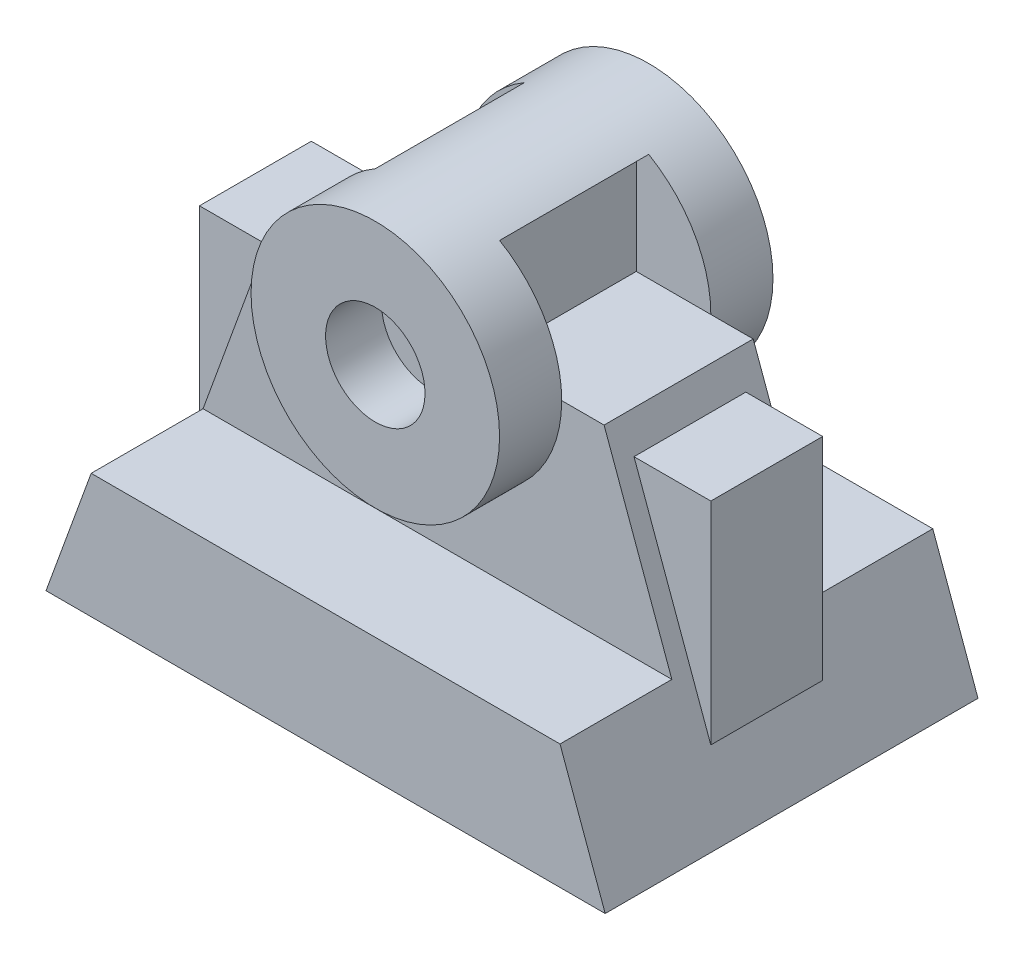
ISO-10303-21;
HEADER;
FILE_DESCRIPTION(('STEP AP214'),'2;1');
FILE_NAME('part.step','',(''),(''),'','','');
FILE_SCHEMA(('AUTOMOTIVE_DESIGN { 1 0 10303 214 1 1 1 1 }'));
ENDSEC;
DATA;
#1=APPLICATION_CONTEXT('core data for automotive mechanical design processes');
#2=APPLICATION_PROTOCOL_DEFINITION('international standard','automotive_design',2000,#1);
#3=PRODUCT_CONTEXT('',#1,'mechanical');
#4=PRODUCT('Part','Part','',(#3));
#5=PRODUCT_RELATED_PRODUCT_CATEGORY('part','',(#4));
#6=PRODUCT_DEFINITION_FORMATION('','',#4);
#7=PRODUCT_DEFINITION_CONTEXT('part definition',#1,'design');
#8=PRODUCT_DEFINITION('design','',#6,#7);
#9=PRODUCT_DEFINITION_SHAPE('','',#8);
#10=(LENGTH_UNIT() NAMED_UNIT(*) SI_UNIT(.MILLI.,.METRE.));
#11=(NAMED_UNIT(*) PLANE_ANGLE_UNIT() SI_UNIT($,.RADIAN.));
#12=(NAMED_UNIT(*) SI_UNIT($,.STERADIAN.) SOLID_ANGLE_UNIT());
#13=UNCERTAINTY_MEASURE_WITH_UNIT(LENGTH_MEASURE(1.E-05),#10,'distance_accuracy_value','');
#14=(GEOMETRIC_REPRESENTATION_CONTEXT(3) GLOBAL_UNCERTAINTY_ASSIGNED_CONTEXT((#13)) GLOBAL_UNIT_ASSIGNED_CONTEXT((#10,
#11,#12)) REPRESENTATION_CONTEXT('',''));
#15=CARTESIAN_POINT('',(0.,0.,0.));
#16=DIRECTION('',(0.,0.,1.));
#17=DIRECTION('',(1.,0.,0.));
#18=AXIS2_PLACEMENT_3D('',#15,#16,#17);
#19=CARTESIAN_POINT('',(45.,50.,7.99999999999999));
#20=DIRECTION('',(0.,0.,1.));
#21=DIRECTION('',(1.,0.,0.));
#22=AXIS2_PLACEMENT_3D('',#19,#20,#21);
#23=CYLINDRICAL_SURFACE('',#22,20.);
#24=CARTESIAN_POINT('',(45.,50.,7.99999999999999));
#25=DIRECTION('',(0.,0.,1.));
#26=DIRECTION('',(1.,0.,0.));
#27=AXIS2_PLACEMENT_3D('',#24,#25,#26);
#28=CIRCLE('',#27,20.);
#29=CARTESIAN_POINT('',(65.,50.,7.99999999999999));
#30=VERTEX_POINT('',#29);
#31=EDGE_CURVE('E315',#30,#30,#28,.T.);
#32=ORIENTED_EDGE('',*,*,#31,.T.);
#33=EDGE_LOOP('',(#32));
#34=FACE_BOUND('',#33,.T.);
#35=CARTESIAN_POINT('',(45.,50.,52.));
#36=DIRECTION('',(0.,0.,1.));
#37=DIRECTION('',(1.,0.,0.));
#38=AXIS2_PLACEMENT_3D('',#35,#36,#37);
#39=CIRCLE('',#38,20.);
#40=CARTESIAN_POINT('',(65.,50.,52.));
#41=VERTEX_POINT('',#40);
#42=EDGE_CURVE('E307',#41,#41,#39,.T.);
#43=ORIENTED_EDGE('',*,*,#42,.F.);
#44=EDGE_LOOP('',(#43));
#45=FACE_BOUND('',#44,.T.);
#46=CARTESIAN_POINT('',(45.,50.,18.));
#47=DIRECTION('',(0.,0.,-1.));
#48=DIRECTION('',(-1.,0.,0.));
#49=AXIS2_PLACEMENT_3D('',#46,#47,#48);
#50=CIRCLE('',#49,20.);
#51=CARTESIAN_POINT('',(65.,50.,18.));
#52=VERTEX_POINT('',#51);
#53=CARTESIAN_POINT('',(25.,50.,18.));
#54=VERTEX_POINT('',#53);
#55=EDGE_CURVE('E320',#52,#54,#50,.T.);
#56=ORIENTED_EDGE('',*,*,#55,.T.);
#57=CARTESIAN_POINT('',(45.,50.,18.));
#58=DIRECTION('',(0.,0.,1.));
#59=DIRECTION('',(1.,0.,0.));
#60=AXIS2_PLACEMENT_3D('',#57,#58,#59);
#61=CIRCLE('',#60,20.);
#62=CARTESIAN_POINT('',(35.,67.3205080756888,18.));
#63=VERTEX_POINT('',#62);
#64=EDGE_CURVE('E11',#54,#63,#61,.F.);
#65=ORIENTED_EDGE('',*,*,#64,.T.);
#66=DIRECTION('',(0.,0.,1.));
#67=VECTOR('',#66,1.);
#68=CARTESIAN_POINT('',(35.,67.3205080756888,7.99999999999999));
#69=LINE('',#68,#67);
#70=CARTESIAN_POINT('',(35.,67.3205080756888,42.));
#71=VERTEX_POINT('',#70);
#72=EDGE_CURVE('E401',#71,#63,#69,.F.);
#73=ORIENTED_EDGE('',*,*,#72,.F.);
#74=CARTESIAN_POINT('',(45.,50.,42.));
#75=DIRECTION('',(0.,0.,-1.));
#76=DIRECTION('',(-1.,0.,0.));
#77=AXIS2_PLACEMENT_3D('',#74,#75,#76);
#78=CIRCLE('',#77,20.);
#79=CARTESIAN_POINT('',(25.,50.,42.));
#80=VERTEX_POINT('',#79);
#81=EDGE_CURVE('E52',#71,#80,#78,.F.);
#82=ORIENTED_EDGE('',*,*,#81,.T.);
#83=CARTESIAN_POINT('',(45.,50.,42.));
#84=DIRECTION('',(0.,0.,1.));
#85=DIRECTION('',(1.,0.,0.));
#86=AXIS2_PLACEMENT_3D('',#83,#84,#85);
#87=CIRCLE('',#86,20.);
#88=CARTESIAN_POINT('',(65.,50.,42.));
#89=VERTEX_POINT('',#88);
#90=EDGE_CURVE('E308',#80,#89,#87,.T.);
#91=ORIENTED_EDGE('',*,*,#90,.T.);
#92=CARTESIAN_POINT('',(45.,50.,42.));
#93=DIRECTION('',(0.,0.,1.));
#94=DIRECTION('',(1.,0.,0.));
#95=AXIS2_PLACEMENT_3D('',#92,#93,#94);
#96=CIRCLE('',#95,20.);
#97=CARTESIAN_POINT('',(55.,67.3205080756888,42.));
#98=VERTEX_POINT('',#97);
#99=EDGE_CURVE('E217',#98,#89,#96,.F.);
#100=ORIENTED_EDGE('',*,*,#99,.F.);
#101=DIRECTION('',(0.,0.,1.));
#102=VECTOR('',#101,1.);
#103=CARTESIAN_POINT('',(55.,67.3205080756888,7.99999999999999));
#104=LINE('',#103,#102);
#105=CARTESIAN_POINT('',(55.,67.3205080756888,18.));
#106=VERTEX_POINT('',#105);
#107=EDGE_CURVE('E396',#106,#98,#104,.T.);
#108=ORIENTED_EDGE('',*,*,#107,.F.);
#109=CARTESIAN_POINT('',(45.,50.,18.));
#110=DIRECTION('',(0.,0.,-1.));
#111=DIRECTION('',(0.,1.,0.));
#112=AXIS2_PLACEMENT_3D('',#109,#110,#111);
#113=CIRCLE('',#112,20.);
#114=EDGE_CURVE('E397',#52,#106,#113,.F.);
#115=ORIENTED_EDGE('',*,*,#114,.F.);
#116=EDGE_LOOP('',(#56,#65,#73,#82,#91,#100,#108,#115));
#117=FACE_BOUND('',#116,.T.);
#118=ADVANCED_FACE('F44',(#34,#45,#117),#23,.T.);
#119=CARTESIAN_POINT('',(20.,55.,18.));
#120=DIRECTION('',(-0.939793423488437,0.341743063086705,0.));
#121=DIRECTION('',(-0.341743063086705,-0.939793423488437,0.));
#122=AXIS2_PLACEMENT_3D('',#119,#120,#121);
#123=PLANE('',#122);
#124=DIRECTION('',(0.,0.,1.));
#125=VECTOR('',#124,1.);
#126=CARTESIAN_POINT('',(18.1818181818182,50.,18.));
#127=LINE('',#126,#125);
#128=CARTESIAN_POINT('',(18.1818181818182,50.,18.));
#129=VERTEX_POINT('',#128);
#130=CARTESIAN_POINT('',(18.1818181818182,50.,42.));
#131=VERTEX_POINT('',#130);
#132=EDGE_CURVE('E342',#129,#131,#127,.T.);
#133=ORIENTED_EDGE('',*,*,#132,.F.);
#134=DIRECTION('',(-0.341743063086705,-0.939793423488437,0.));
#135=VECTOR('',#134,1.);
#136=CARTESIAN_POINT('',(20.,55.,18.));
#137=LINE('',#136,#135);
#138=CARTESIAN_POINT('',(7.27272727272728,20.,18.));
#139=VERTEX_POINT('',#138);
#140=EDGE_CURVE('E364',#129,#139,#137,.T.);
#141=ORIENTED_EDGE('',*,*,#140,.T.);
#142=DIRECTION('',(0.,0.,1.));
#143=VECTOR('',#142,1.);
#144=CARTESIAN_POINT('',(7.27272727272728,20.,0.));
#145=LINE('',#144,#143);
#146=CARTESIAN_POINT('',(7.27272727272728,20.,0.));
#147=VERTEX_POINT('',#146);
#148=EDGE_CURVE('E328',#147,#139,#145,.T.);
#149=ORIENTED_EDGE('',*,*,#148,.F.);
#150=DIRECTION('',(-0.341743063086704,-0.939793423488437,0.));
#151=VECTOR('',#150,1.);
#152=CARTESIAN_POINT('',(0.,0.,0.));
#153=LINE('',#152,#151);
#154=CARTESIAN_POINT('',(0.,0.,0.));
#155=VERTEX_POINT('',#154);
#156=EDGE_CURVE('E323',#147,#155,#153,.T.);
#157=ORIENTED_EDGE('',*,*,#156,.T.);
#158=DIRECTION('',(0.,0.,-1.));
#159=VECTOR('',#158,1.);
#160=CARTESIAN_POINT('',(0.,0.,60.));
#161=LINE('',#160,#159);
#162=CARTESIAN_POINT('',(0.,0.,60.));
#163=VERTEX_POINT('',#162);
#164=EDGE_CURVE('E382',#163,#155,#161,.T.);
#165=ORIENTED_EDGE('',*,*,#164,.F.);
#166=DIRECTION('',(-0.341743063086704,-0.939793423488437,0.));
#167=VECTOR('',#166,1.);
#168=CARTESIAN_POINT('',(0.,0.,60.));
#169=LINE('',#168,#167);
#170=CARTESIAN_POINT('',(7.27272727272728,20.,60.));
#171=VERTEX_POINT('',#170);
#172=EDGE_CURVE('E324',#171,#163,#169,.T.);
#173=ORIENTED_EDGE('',*,*,#172,.F.);
#174=CARTESIAN_POINT('',(7.27272727272728,20.,42.));
#175=VERTEX_POINT('',#174);
#176=EDGE_CURVE('E321',#175,#171,#145,.T.);
#177=ORIENTED_EDGE('',*,*,#176,.F.);
#178=DIRECTION('',(-0.341743063086705,-0.939793423488437,0.));
#179=VECTOR('',#178,1.);
#180=CARTESIAN_POINT('',(7.27272727272728,20.,42.));
#181=LINE('',#180,#179);
#182=EDGE_CURVE('E354',#131,#175,#181,.T.);
#183=ORIENTED_EDGE('',*,*,#182,.F.);
#184=EDGE_LOOP('',(#133,#141,#149,#157,#165,#173,#177,#183));
#185=FACE_BOUND('',#184,.T.);
#186=DIRECTION('',(0.341743063086705,0.939793423488437,0.));
#187=VECTOR('',#186,1.);
#188=CARTESIAN_POINT('',(20.,55.,21.));
#189=LINE('',#188,#187);
#190=CARTESIAN_POINT('',(3.63636363636363,9.99999999999999,21.));
#191=VERTEX_POINT('',#190);
#192=CARTESIAN_POINT('',(3.7,10.175,21.));
#193=VERTEX_POINT('',#192);
#194=EDGE_CURVE('E301',#191,#193,#189,.T.);
#195=ORIENTED_EDGE('',*,*,#194,.T.);
#196=CARTESIAN_POINT('',(16.3636363636364,45.,21.));
#197=VERTEX_POINT('',#196);
#198=EDGE_CURVE('E68',#193,#197,#189,.T.);
#199=ORIENTED_EDGE('',*,*,#198,.T.);
#200=DIRECTION('',(0.,0.,1.));
#201=VECTOR('',#200,1.);
#202=CARTESIAN_POINT('',(16.3636363636364,45.,18.));
#203=LINE('',#202,#201);
#204=CARTESIAN_POINT('',(16.3636363636364,45.,39.));
#205=VERTEX_POINT('',#204);
#206=EDGE_CURVE('E306',#197,#205,#203,.T.);
#207=ORIENTED_EDGE('',*,*,#206,.T.);
#208=DIRECTION('',(-0.341743063086705,-0.939793423488437,0.));
#209=VECTOR('',#208,1.);
#210=CARTESIAN_POINT('',(20.,55.,39.));
#211=LINE('',#210,#209);
#212=CARTESIAN_POINT('',(3.7,10.175,39.));
#213=VERTEX_POINT('',#212);
#214=EDGE_CURVE('E303',#205,#213,#211,.T.);
#215=ORIENTED_EDGE('',*,*,#214,.T.);
#216=DIRECTION('',(0.341743063086705,0.939793423488437,0.));
#217=VECTOR('',#216,1.);
#218=CARTESIAN_POINT('',(20.,55.,39.));
#219=LINE('',#218,#217);
#220=CARTESIAN_POINT('',(3.63636363636363,9.99999999999999,39.));
#221=VERTEX_POINT('',#220);
#222=EDGE_CURVE('E285',#221,#213,#219,.T.);
#223=ORIENTED_EDGE('',*,*,#222,.F.);
#224=DIRECTION('',(0.,0.,-1.));
#225=VECTOR('',#224,1.);
#226=CARTESIAN_POINT('',(3.63636363636363,9.99999999999999,18.));
#227=LINE('',#226,#225);
#228=EDGE_CURVE('E393',#221,#191,#227,.T.);
#229=ORIENTED_EDGE('',*,*,#228,.T.);
#230=EDGE_LOOP('',(#195,#199,#207,#215,#223,#229));
#231=FACE_BOUND('',#230,.T.);
#232=ADVANCED_FACE('F440',(#185,#231),#123,.T.);
#233=CARTESIAN_POINT('',(70.,55.,18.));
#234=DIRECTION('',(0.939793423488437,0.341743063086704,0.));
#235=DIRECTION('',(-0.341743063086704,0.939793423488437,0.));
#236=AXIS2_PLACEMENT_3D('',#233,#234,#235);
#237=PLANE('',#236);
#238=DIRECTION('',(0.,0.,1.));
#239=VECTOR('',#238,1.);
#240=CARTESIAN_POINT('',(71.8181818181818,50.,18.));
#241=LINE('',#240,#239);
#242=CARTESIAN_POINT('',(71.8181818181818,50.,18.));
#243=VERTEX_POINT('',#242);
#244=CARTESIAN_POINT('',(71.8181818181818,50.,42.));
#245=VERTEX_POINT('',#244);
#246=EDGE_CURVE('E338',#243,#245,#241,.T.);
#247=ORIENTED_EDGE('',*,*,#246,.T.);
#248=DIRECTION('',(-0.341743063086704,0.939793423488437,0.));
#249=VECTOR('',#248,1.);
#250=CARTESIAN_POINT('',(70.,55.,42.));
#251=LINE('',#250,#249);
#252=CARTESIAN_POINT('',(82.7272727272727,20.,42.));
#253=VERTEX_POINT('',#252);
#254=EDGE_CURVE('E355',#253,#245,#251,.T.);
#255=ORIENTED_EDGE('',*,*,#254,.F.);
#256=DIRECTION('',(0.,0.,1.));
#257=VECTOR('',#256,1.);
#258=CARTESIAN_POINT('',(82.7272727272727,20.,0.));
#259=LINE('',#258,#257);
#260=CARTESIAN_POINT('',(82.7272727272727,20.,60.));
#261=VERTEX_POINT('',#260);
#262=EDGE_CURVE('E332',#253,#261,#259,.T.);
#263=ORIENTED_EDGE('',*,*,#262,.T.);
#264=DIRECTION('',(0.341743063086704,-0.939793423488437,0.));
#265=VECTOR('',#264,1.);
#266=CARTESIAN_POINT('',(79.4890510948905,28.9051094890511,60.));
#267=LINE('',#266,#265);
#268=CARTESIAN_POINT('',(90.,0.,60.));
#269=VERTEX_POINT('',#268);
#270=EDGE_CURVE('E318',#261,#269,#267,.T.);
#271=ORIENTED_EDGE('',*,*,#270,.T.);
#272=DIRECTION('',(0.,0.,-1.));
#273=VECTOR('',#272,1.);
#274=CARTESIAN_POINT('',(90.,0.,60.));
#275=LINE('',#274,#273);
#276=CARTESIAN_POINT('',(90.,0.,0.));
#277=VERTEX_POINT('',#276);
#278=EDGE_CURVE('E374',#269,#277,#275,.T.);
#279=ORIENTED_EDGE('',*,*,#278,.T.);
#280=DIRECTION('',(0.341743063086704,-0.939793423488437,0.));
#281=VECTOR('',#280,1.);
#282=CARTESIAN_POINT('',(79.4890510948905,28.9051094890511,0.));
#283=LINE('',#282,#281);
#284=CARTESIAN_POINT('',(82.7272727272727,20.,0.));
#285=VERTEX_POINT('',#284);
#286=EDGE_CURVE('E331',#285,#277,#283,.T.);
#287=ORIENTED_EDGE('',*,*,#286,.F.);
#288=CARTESIAN_POINT('',(82.7272727272727,20.,18.));
#289=VERTEX_POINT('',#288);
#290=EDGE_CURVE('E330',#285,#289,#259,.T.);
#291=ORIENTED_EDGE('',*,*,#290,.T.);
#292=DIRECTION('',(-0.341743063086704,0.939793423488437,0.));
#293=VECTOR('',#292,1.);
#294=CARTESIAN_POINT('',(70.,55.,18.));
#295=LINE('',#294,#293);
#296=EDGE_CURVE('E363',#289,#243,#295,.T.);
#297=ORIENTED_EDGE('',*,*,#296,.T.);
#298=EDGE_LOOP('',(#247,#255,#263,#271,#279,#287,#291,#297));
#299=FACE_BOUND('',#298,.T.);
#300=DIRECTION('',(-0.341743063086704,0.939793423488437,0.));
#301=VECTOR('',#300,1.);
#302=CARTESIAN_POINT('',(70.,55.,39.));
#303=LINE('',#302,#301);
#304=CARTESIAN_POINT('',(86.,11.,39.));
#305=VERTEX_POINT('',#304);
#306=CARTESIAN_POINT('',(73.6363636363637,45.,39.));
#307=VERTEX_POINT('',#306);
#308=EDGE_CURVE('E389',#305,#307,#303,.T.);
#309=ORIENTED_EDGE('',*,*,#308,.T.);
#310=DIRECTION('',(0.,0.,-1.));
#311=VECTOR('',#310,1.);
#312=CARTESIAN_POINT('',(73.6363636363637,45.,18.));
#313=LINE('',#312,#311);
#314=CARTESIAN_POINT('',(73.6363636363637,45.,21.));
#315=VERTEX_POINT('',#314);
#316=EDGE_CURVE('E392',#307,#315,#313,.T.);
#317=ORIENTED_EDGE('',*,*,#316,.T.);
#318=DIRECTION('',(0.341743063086704,-0.939793423488437,0.));
#319=VECTOR('',#318,1.);
#320=CARTESIAN_POINT('',(70.,55.,21.));
#321=LINE('',#320,#319);
#322=CARTESIAN_POINT('',(86.,11.,21.));
#323=VERTEX_POINT('',#322);
#324=EDGE_CURVE('E390',#315,#323,#321,.T.);
#325=ORIENTED_EDGE('',*,*,#324,.T.);
#326=DIRECTION('',(0.,0.,-1.));
#327=VECTOR('',#326,1.);
#328=CARTESIAN_POINT('',(86.,11.,18.));
#329=LINE('',#328,#327);
#330=EDGE_CURVE('E381',#305,#323,#329,.T.);
#331=ORIENTED_EDGE('',*,*,#330,.F.);
#332=EDGE_LOOP('',(#309,#317,#325,#331));
#333=FACE_BOUND('',#332,.T.);
#334=ADVANCED_FACE('F421',(#299,#333),#237,.T.);
#335=CARTESIAN_POINT('',(0.,0.,42.));
#336=DIRECTION('',(0.,0.,-1.));
#337=DIRECTION('',(-1.,0.,0.));
#338=AXIS2_PLACEMENT_3D('',#335,#336,#337);
#339=PLANE('',#338);
#340=ORIENTED_EDGE('',*,*,#90,.F.);
#341=DIRECTION('',(1.,0.,0.));
#342=VECTOR('',#341,1.);
#343=CARTESIAN_POINT('',(45.,50.,42.));
#344=LINE('',#343,#342);
#345=EDGE_CURVE('E345',#131,#80,#344,.T.);
#346=ORIENTED_EDGE('',*,*,#345,.F.);
#347=ORIENTED_EDGE('',*,*,#182,.T.);
#348=DIRECTION('',(1.,0.,0.));
#349=VECTOR('',#348,1.);
#350=CARTESIAN_POINT('',(82.7272727272727,20.,42.));
#351=LINE('',#350,#349);
#352=EDGE_CURVE('E350',#175,#253,#351,.T.);
#353=ORIENTED_EDGE('',*,*,#352,.T.);
#354=ORIENTED_EDGE('',*,*,#254,.T.);
#355=EDGE_CURVE('E326',#89,#245,#344,.T.);
#356=ORIENTED_EDGE('',*,*,#355,.F.);
#357=EDGE_LOOP('',(#340,#346,#347,#353,#354,#356));
#358=FACE_BOUND('',#357,.T.);
#359=ADVANCED_FACE('F417',(#358),#339,.F.);
#360=CARTESIAN_POINT('',(45.,50.,18.));
#361=DIRECTION('',(0.,-1.,0.));
#362=DIRECTION('',(0.,0.,-1.));
#363=AXIS2_PLACEMENT_3D('',#360,#361,#362);
#364=PLANE('',#363);
#365=DIRECTION('',(1.,0.,0.));
#366=VECTOR('',#365,1.);
#367=CARTESIAN_POINT('',(45.,50.,18.));
#368=LINE('',#367,#366);
#369=EDGE_CURVE('E343',#52,#243,#368,.T.);
#370=ORIENTED_EDGE('',*,*,#369,.F.);
#371=DIRECTION('',(1.,0.,0.));
#372=VECTOR('',#371,1.);
#373=CARTESIAN_POINT('',(55.,50.,18.));
#374=LINE('',#373,#372);
#375=CARTESIAN_POINT('',(53.,50.,18.));
#376=VERTEX_POINT('',#375);
#377=EDGE_CURVE('E219',#376,#52,#374,.T.);
#378=ORIENTED_EDGE('',*,*,#377,.F.);
#379=DIRECTION('',(0.,0.,-1.));
#380=VECTOR('',#379,1.);
#381=CARTESIAN_POINT('',(53.,50.,18.));
#382=LINE('',#381,#380);
#383=CARTESIAN_POINT('',(53.,50.,42.));
#384=VERTEX_POINT('',#383);
#385=EDGE_CURVE('E223',#384,#376,#382,.T.);
#386=ORIENTED_EDGE('',*,*,#385,.F.);
#387=DIRECTION('',(1.,0.,0.));
#388=VECTOR('',#387,1.);
#389=CARTESIAN_POINT('',(55.,50.,42.));
#390=LINE('',#389,#388);
#391=EDGE_CURVE('E209',#384,#89,#390,.T.);
#392=ORIENTED_EDGE('',*,*,#391,.T.);
#393=ORIENTED_EDGE('',*,*,#355,.T.);
#394=ORIENTED_EDGE('',*,*,#246,.F.);
#395=EDGE_LOOP('',(#370,#378,#386,#392,#393,#394));
#396=FACE_BOUND('',#395,.T.);
#397=ADVANCED_FACE('F224',(#396),#364,.F.);
#398=CARTESIAN_POINT('',(90.,20.,60.));
#399=DIRECTION('',(0.,-1.,0.));
#400=DIRECTION('',(0.,0.,-1.));
#401=AXIS2_PLACEMENT_3D('',#398,#399,#400);
#402=PLANE('',#401);
#403=ORIENTED_EDGE('',*,*,#176,.T.);
#404=DIRECTION('',(-1.,0.,0.));
#405=VECTOR('',#404,1.);
#406=CARTESIAN_POINT('',(90.,20.,60.));
#407=LINE('',#406,#405);
#408=EDGE_CURVE('E371',#261,#171,#407,.T.);
#409=ORIENTED_EDGE('',*,*,#408,.F.);
#410=ORIENTED_EDGE('',*,*,#262,.F.);
#411=ORIENTED_EDGE('',*,*,#352,.F.);
#412=EDGE_LOOP('',(#403,#409,#410,#411));
#413=FACE_BOUND('',#412,.T.);
#414=ADVANCED_FACE('F484',(#413),#402,.F.);
#415=ORIENTED_EDGE('',*,*,#148,.T.);
#416=DIRECTION('',(1.,0.,0.));
#417=VECTOR('',#416,1.);
#418=CARTESIAN_POINT('',(45.,20.,18.));
#419=LINE('',#418,#417);
#420=EDGE_CURVE('E356',#139,#289,#419,.T.);
#421=ORIENTED_EDGE('',*,*,#420,.T.);
#422=ORIENTED_EDGE('',*,*,#290,.F.);
#423=DIRECTION('',(-1.,0.,0.));
#424=VECTOR('',#423,1.);
#425=CARTESIAN_POINT('',(90.,20.,0.));
#426=LINE('',#425,#424);
#427=EDGE_CURVE('E375',#285,#147,#426,.T.);
#428=ORIENTED_EDGE('',*,*,#427,.T.);
#429=EDGE_LOOP('',(#415,#421,#422,#428));
#430=FACE_BOUND('',#429,.T.);
#431=ADVANCED_FACE('F433',(#430),#402,.F.);
#432=CARTESIAN_POINT('',(0.,0.,60.));
#433=DIRECTION('',(0.,0.,1.));
#434=DIRECTION('',(1.,0.,0.));
#435=AXIS2_PLACEMENT_3D('',#432,#433,#434);
#436=PLANE('',#435);
#437=ORIENTED_EDGE('',*,*,#408,.T.);
#438=ORIENTED_EDGE('',*,*,#172,.T.);
#439=DIRECTION('',(1.,0.,0.));
#440=VECTOR('',#439,1.);
#441=CARTESIAN_POINT('',(0.,0.,60.));
#442=LINE('',#441,#440);
#443=EDGE_CURVE('E368',#163,#269,#442,.T.);
#444=ORIENTED_EDGE('',*,*,#443,.T.);
#445=ORIENTED_EDGE('',*,*,#270,.F.);
#446=EDGE_LOOP('',(#437,#438,#444,#445));
#447=FACE_BOUND('',#446,.T.);
#448=ADVANCED_FACE('F478',(#447),#436,.T.);
#449=CARTESIAN_POINT('',(0.,0.,0.));
#450=DIRECTION('',(0.,0.,1.));
#451=DIRECTION('',(1.,0.,0.));
#452=AXIS2_PLACEMENT_3D('',#449,#450,#451);
#453=PLANE('',#452);
#454=ORIENTED_EDGE('',*,*,#156,.F.);
#455=ORIENTED_EDGE('',*,*,#427,.F.);
#456=ORIENTED_EDGE('',*,*,#286,.T.);
#457=DIRECTION('',(1.,0.,0.));
#458=VECTOR('',#457,1.);
#459=CARTESIAN_POINT('',(0.,0.,0.));
#460=LINE('',#459,#458);
#461=EDGE_CURVE('E370',#155,#277,#460,.T.);
#462=ORIENTED_EDGE('',*,*,#461,.F.);
#463=EDGE_LOOP('',(#454,#455,#456,#462));
#464=FACE_BOUND('',#463,.T.);
#465=ADVANCED_FACE('F481',(#464),#453,.F.);
#466=CARTESIAN_POINT('',(0.,0.,60.));
#467=DIRECTION('',(0.,1.,0.));
#468=DIRECTION('',(0.,0.,1.));
#469=AXIS2_PLACEMENT_3D('',#466,#467,#468);
#470=PLANE('',#469);
#471=ORIENTED_EDGE('',*,*,#461,.T.);
#472=ORIENTED_EDGE('',*,*,#278,.F.);
#473=ORIENTED_EDGE('',*,*,#443,.F.);
#474=ORIENTED_EDGE('',*,*,#164,.T.);
#475=EDGE_LOOP('',(#471,#472,#473,#474));
#476=FACE_BOUND('',#475,.T.);
#477=ADVANCED_FACE('F50',(#476),#470,.F.);
#478=CARTESIAN_POINT('',(0.,0.,18.));
#479=DIRECTION('',(0.,0.,-1.));
#480=DIRECTION('',(-1.,0.,0.));
#481=AXIS2_PLACEMENT_3D('',#478,#479,#480);
#482=PLANE('',#481);
#483=ORIENTED_EDGE('',*,*,#55,.F.);
#484=ORIENTED_EDGE('',*,*,#369,.T.);
#485=ORIENTED_EDGE('',*,*,#296,.F.);
#486=ORIENTED_EDGE('',*,*,#420,.F.);
#487=ORIENTED_EDGE('',*,*,#140,.F.);
#488=EDGE_CURVE('E340',#129,#54,#368,.T.);
#489=ORIENTED_EDGE('',*,*,#488,.T.);
#490=EDGE_LOOP('',(#483,#484,#485,#486,#487,#489));
#491=FACE_BOUND('',#490,.T.);
#492=ADVANCED_FACE('F427',(#491),#482,.T.);
#493=ORIENTED_EDGE('',*,*,#345,.T.);
#494=DIRECTION('',(-1.,0.,0.));
#495=VECTOR('',#494,1.);
#496=CARTESIAN_POINT('',(35.,50.,42.));
#497=LINE('',#496,#495);
#498=CARTESIAN_POINT('',(37.,50.,42.));
#499=VERTEX_POINT('',#498);
#500=EDGE_CURVE('E265',#499,#80,#497,.T.);
#501=ORIENTED_EDGE('',*,*,#500,.F.);
#502=DIRECTION('',(0.,0.,1.));
#503=VECTOR('',#502,1.);
#504=CARTESIAN_POINT('',(37.,50.,42.));
#505=LINE('',#504,#503);
#506=CARTESIAN_POINT('',(37.,50.,18.));
#507=VERTEX_POINT('',#506);
#508=EDGE_CURVE('E249',#507,#499,#505,.T.);
#509=ORIENTED_EDGE('',*,*,#508,.F.);
#510=DIRECTION('',(-1.,0.,0.));
#511=VECTOR('',#510,1.);
#512=CARTESIAN_POINT('',(35.,50.,18.));
#513=LINE('',#512,#511);
#514=EDGE_CURVE('E216',#507,#54,#513,.T.);
#515=ORIENTED_EDGE('',*,*,#514,.T.);
#516=ORIENTED_EDGE('',*,*,#488,.F.);
#517=ORIENTED_EDGE('',*,*,#132,.T.);
#518=EDGE_LOOP('',(#493,#501,#509,#515,#516,#517));
#519=FACE_BOUND('',#518,.T.);
#520=ADVANCED_FACE('F413',(#519),#364,.F.);
#521=CARTESIAN_POINT('',(45.,50.,7.99999999999999));
#522=DIRECTION('',(0.,0.,1.));
#523=DIRECTION('',(1.,0.,0.));
#524=AXIS2_PLACEMENT_3D('',#521,#522,#523);
#525=PLANE('',#524);
#526=CARTESIAN_POINT('',(45.,50.,7.99999999999999));
#527=DIRECTION('',(0.,0.,-1.));
#528=DIRECTION('',(-1.,0.,0.));
#529=AXIS2_PLACEMENT_3D('',#526,#527,#528);
#530=CIRCLE('',#529,8.00000000000001);
#531=CARTESIAN_POINT('',(37.,50.,7.99999999999999));
#532=VERTEX_POINT('',#531);
#533=EDGE_CURVE('E908',#532,#532,#530,.T.);
#534=ORIENTED_EDGE('',*,*,#533,.F.);
#535=EDGE_LOOP('',(#534));
#536=FACE_BOUND('',#535,.T.);
#537=ORIENTED_EDGE('',*,*,#31,.F.);
#538=EDGE_LOOP('',(#537));
#539=FACE_BOUND('',#538,.T.);
#540=ADVANCED_FACE('F466',(#536,#539),#525,.F.);
#541=CARTESIAN_POINT('',(45.,50.,52.));
#542=DIRECTION('',(0.,0.,1.));
#543=DIRECTION('',(1.,0.,0.));
#544=AXIS2_PLACEMENT_3D('',#541,#542,#543);
#545=PLANE('',#544);
#546=CARTESIAN_POINT('',(45.,50.,52.));
#547=DIRECTION('',(0.,0.,1.));
#548=DIRECTION('',(1.,0.,0.));
#549=AXIS2_PLACEMENT_3D('',#546,#547,#548);
#550=CIRCLE('',#549,8.);
#551=CARTESIAN_POINT('',(53.,50.,52.));
#552=VERTEX_POINT('',#551);
#553=EDGE_CURVE('E240',#552,#552,#550,.T.);
#554=ORIENTED_EDGE('',*,*,#553,.F.);
#555=EDGE_LOOP('',(#554));
#556=FACE_BOUND('',#555,.T.);
#557=ORIENTED_EDGE('',*,*,#42,.T.);
#558=EDGE_LOOP('',(#557));
#559=FACE_BOUND('',#558,.T.);
#560=ADVANCED_FACE('F523',(#556,#559),#545,.T.);
#561=CARTESIAN_POINT('',(86.,0.,0.));
#562=DIRECTION('',(1.,0.,0.));
#563=DIRECTION('',(0.,0.,-1.));
#564=AXIS2_PLACEMENT_3D('',#561,#562,#563);
#565=PLANE('',#564);
#566=DIRECTION('',(0.,-1.,0.));
#567=VECTOR('',#566,1.);
#568=CARTESIAN_POINT('',(86.,45.,39.));
#569=LINE('',#568,#567);
#570=CARTESIAN_POINT('',(86.,45.,39.));
#571=VERTEX_POINT('',#570);
#572=EDGE_CURVE('E288',#571,#305,#569,.T.);
#573=ORIENTED_EDGE('',*,*,#572,.T.);
#574=ORIENTED_EDGE('',*,*,#330,.T.);
#575=DIRECTION('',(0.,1.,0.));
#576=VECTOR('',#575,1.);
#577=CARTESIAN_POINT('',(86.,9.99999999999999,21.));
#578=LINE('',#577,#576);
#579=CARTESIAN_POINT('',(86.,45.,21.));
#580=VERTEX_POINT('',#579);
#581=EDGE_CURVE('E293',#323,#580,#578,.T.);
#582=ORIENTED_EDGE('',*,*,#581,.T.);
#583=DIRECTION('',(0.,0.,1.));
#584=VECTOR('',#583,1.);
#585=CARTESIAN_POINT('',(86.,45.,21.));
#586=LINE('',#585,#584);
#587=EDGE_CURVE('E286',#580,#571,#586,.T.);
#588=ORIENTED_EDGE('',*,*,#587,.T.);
#589=EDGE_LOOP('',(#573,#574,#582,#588));
#590=FACE_BOUND('',#589,.T.);
#591=ADVANCED_FACE('F518',(#590),#565,.T.);
#592=CARTESIAN_POINT('',(86.,9.99999999999999,21.));
#593=DIRECTION('',(0.,0.,1.));
#594=DIRECTION('',(1.,0.,0.));
#595=AXIS2_PLACEMENT_3D('',#592,#593,#594);
#596=PLANE('',#595);
#597=ORIENTED_EDGE('',*,*,#324,.F.);
#598=DIRECTION('',(-1.,0.,0.));
#599=VECTOR('',#598,1.);
#600=CARTESIAN_POINT('',(86.,45.,21.));
#601=LINE('',#600,#599);
#602=EDGE_CURVE('E295',#580,#315,#601,.T.);
#603=ORIENTED_EDGE('',*,*,#602,.F.);
#604=ORIENTED_EDGE('',*,*,#581,.F.);
#605=EDGE_LOOP('',(#597,#603,#604));
#606=FACE_BOUND('',#605,.T.);
#607=ADVANCED_FACE('F525',(#606),#596,.F.);
#608=CARTESIAN_POINT('',(86.,45.,39.));
#609=DIRECTION('',(0.,0.,-1.));
#610=DIRECTION('',(-1.,0.,0.));
#611=AXIS2_PLACEMENT_3D('',#608,#609,#610);
#612=PLANE('',#611);
#613=ORIENTED_EDGE('',*,*,#308,.F.);
#614=ORIENTED_EDGE('',*,*,#572,.F.);
#615=DIRECTION('',(-1.,0.,0.));
#616=VECTOR('',#615,1.);
#617=CARTESIAN_POINT('',(86.,45.,39.));
#618=LINE('',#617,#616);
#619=EDGE_CURVE('E296',#571,#307,#618,.T.);
#620=ORIENTED_EDGE('',*,*,#619,.T.);
#621=EDGE_LOOP('',(#613,#614,#620));
#622=FACE_BOUND('',#621,.T.);
#623=ADVANCED_FACE('F540',(#622),#612,.F.);
#624=CARTESIAN_POINT('',(86.,45.,30.));
#625=DIRECTION('',(0.,-1.,0.));
#626=DIRECTION('',(0.,0.,-1.));
#627=AXIS2_PLACEMENT_3D('',#624,#625,#626);
#628=PLANE('',#627);
#629=ORIENTED_EDGE('',*,*,#316,.F.);
#630=ORIENTED_EDGE('',*,*,#619,.F.);
#631=ORIENTED_EDGE('',*,*,#587,.F.);
#632=ORIENTED_EDGE('',*,*,#602,.T.);
#633=EDGE_LOOP('',(#629,#630,#631,#632));
#634=FACE_BOUND('',#633,.T.);
#635=ADVANCED_FACE('F549',(#634),#628,.F.);
#636=CARTESIAN_POINT('',(3.69999999999999,45.,21.));
#637=VERTEX_POINT('',#636);
#638=EDGE_CURVE('E291',#197,#637,#601,.T.);
#639=ORIENTED_EDGE('',*,*,#638,.T.);
#640=DIRECTION('',(0.,0.,-1.));
#641=VECTOR('',#640,1.);
#642=CARTESIAN_POINT('',(3.7,45.,21.));
#643=LINE('',#642,#641);
#644=CARTESIAN_POINT('',(3.7,45.,39.));
#645=VERTEX_POINT('',#644);
#646=EDGE_CURVE('E58',#645,#637,#643,.T.);
#647=ORIENTED_EDGE('',*,*,#646,.F.);
#648=EDGE_CURVE('E300',#205,#645,#618,.T.);
#649=ORIENTED_EDGE('',*,*,#648,.F.);
#650=ORIENTED_EDGE('',*,*,#206,.F.);
#651=EDGE_LOOP('',(#639,#647,#649,#650));
#652=FACE_BOUND('',#651,.T.);
#653=ADVANCED_FACE('F563',(#652),#628,.F.);
#654=ORIENTED_EDGE('',*,*,#648,.T.);
#655=DIRECTION('',(0.,1.,0.));
#656=VECTOR('',#655,1.);
#657=CARTESIAN_POINT('',(3.7,45.,39.));
#658=LINE('',#657,#656);
#659=EDGE_CURVE('E271',#213,#645,#658,.T.);
#660=ORIENTED_EDGE('',*,*,#659,.F.);
#661=ORIENTED_EDGE('',*,*,#214,.F.);
#662=EDGE_LOOP('',(#654,#660,#661));
#663=FACE_BOUND('',#662,.T.);
#664=ADVANCED_FACE('F551',(#663),#612,.F.);
#665=ORIENTED_EDGE('',*,*,#198,.F.);
#666=DIRECTION('',(0.,-1.,0.));
#667=VECTOR('',#666,1.);
#668=CARTESIAN_POINT('',(3.7,9.99999999999999,21.));
#669=LINE('',#668,#667);
#670=EDGE_CURVE('E268',#637,#193,#669,.T.);
#671=ORIENTED_EDGE('',*,*,#670,.F.);
#672=ORIENTED_EDGE('',*,*,#638,.F.);
#673=EDGE_LOOP('',(#665,#671,#672));
#674=FACE_BOUND('',#673,.T.);
#675=ADVANCED_FACE('F537',(#674),#596,.F.);
#676=CARTESIAN_POINT('',(3.7,9.99999999999999,21.));
#677=DIRECTION('',(0.,0.,-1.));
#678=DIRECTION('',(-1.,0.,0.));
#679=AXIS2_PLACEMENT_3D('',#676,#677,#678);
#680=PLANE('',#679);
#681=ORIENTED_EDGE('',*,*,#194,.F.);
#682=DIRECTION('',(-1.,0.,0.));
#683=VECTOR('',#682,1.);
#684=CARTESIAN_POINT('',(3.7,9.99999999999999,21.));
#685=LINE('',#684,#683);
#686=CARTESIAN_POINT('',(3.7,9.99999999999999,21.));
#687=VERTEX_POINT('',#686);
#688=EDGE_CURVE('E276',#687,#191,#685,.T.);
#689=ORIENTED_EDGE('',*,*,#688,.F.);
#690=EDGE_CURVE('E266',#193,#687,#669,.T.);
#691=ORIENTED_EDGE('',*,*,#690,.F.);
#692=EDGE_LOOP('',(#681,#689,#691));
#693=FACE_BOUND('',#692,.T.);
#694=ADVANCED_FACE('F600',(#693),#680,.F.);
#695=CARTESIAN_POINT('',(3.7,45.,39.));
#696=DIRECTION('',(0.,0.,1.));
#697=DIRECTION('',(1.,0.,0.));
#698=AXIS2_PLACEMENT_3D('',#695,#696,#697);
#699=PLANE('',#698);
#700=ORIENTED_EDGE('',*,*,#222,.T.);
#701=CARTESIAN_POINT('',(3.7,9.99999999999999,39.));
#702=VERTEX_POINT('',#701);
#703=EDGE_CURVE('E274',#702,#213,#658,.T.);
#704=ORIENTED_EDGE('',*,*,#703,.F.);
#705=DIRECTION('',(-1.,0.,0.));
#706=VECTOR('',#705,1.);
#707=CARTESIAN_POINT('',(3.7,9.99999999999999,39.));
#708=LINE('',#707,#706);
#709=EDGE_CURVE('E279',#702,#221,#708,.T.);
#710=ORIENTED_EDGE('',*,*,#709,.T.);
#711=EDGE_LOOP('',(#700,#704,#710));
#712=FACE_BOUND('',#711,.T.);
#713=ADVANCED_FACE('F610',(#712),#699,.F.);
#714=CARTESIAN_POINT('',(3.7,9.99999999999999,39.));
#715=DIRECTION('',(0.,-1.,0.));
#716=DIRECTION('',(0.,0.,-1.));
#717=AXIS2_PLACEMENT_3D('',#714,#715,#716);
#718=PLANE('',#717);
#719=ORIENTED_EDGE('',*,*,#228,.F.);
#720=ORIENTED_EDGE('',*,*,#709,.F.);
#721=DIRECTION('',(0.,0.,1.));
#722=VECTOR('',#721,1.);
#723=CARTESIAN_POINT('',(3.7,9.99999999999999,39.));
#724=LINE('',#723,#722);
#725=EDGE_CURVE('E269',#687,#702,#724,.T.);
#726=ORIENTED_EDGE('',*,*,#725,.F.);
#727=ORIENTED_EDGE('',*,*,#688,.T.);
#728=EDGE_LOOP('',(#719,#720,#726,#727));
#729=FACE_BOUND('',#728,.T.);
#730=ADVANCED_FACE('F618',(#729),#718,.F.);
#731=CARTESIAN_POINT('',(3.7,0.,0.));
#732=DIRECTION('',(1.,0.,0.));
#733=DIRECTION('',(0.,0.,-1.));
#734=AXIS2_PLACEMENT_3D('',#731,#732,#733);
#735=PLANE('',#734);
#736=ORIENTED_EDGE('',*,*,#670,.T.);
#737=ORIENTED_EDGE('',*,*,#690,.T.);
#738=ORIENTED_EDGE('',*,*,#725,.T.);
#739=ORIENTED_EDGE('',*,*,#703,.T.);
#740=ORIENTED_EDGE('',*,*,#659,.T.);
#741=ORIENTED_EDGE('',*,*,#646,.T.);
#742=EDGE_LOOP('',(#736,#737,#738,#739,#740,#741));
#743=FACE_BOUND('',#742,.T.);
#744=ADVANCED_FACE('F622',(#743),#735,.F.);
#745=CARTESIAN_POINT('',(55.,70.,42.));
#746=DIRECTION('',(0.,0.,1.));
#747=DIRECTION('',(1.,0.,0.));
#748=AXIS2_PLACEMENT_3D('',#745,#746,#747);
#749=PLANE('',#748);
#750=ORIENTED_EDGE('',*,*,#99,.T.);
#751=ORIENTED_EDGE('',*,*,#391,.F.);
#752=DIRECTION('',(0.,-1.,0.));
#753=VECTOR('',#752,1.);
#754=CARTESIAN_POINT('',(53.,50.,42.));
#755=LINE('',#754,#753);
#756=CARTESIAN_POINT('',(53.,67.3205080756888,42.));
#757=VERTEX_POINT('',#756);
#758=EDGE_CURVE('E211',#757,#384,#755,.T.);
#759=ORIENTED_EDGE('',*,*,#758,.F.);
#760=DIRECTION('',(1.,0.,0.));
#761=VECTOR('',#760,1.);
#762=CARTESIAN_POINT('',(53.,67.3205080756888,42.));
#763=LINE('',#762,#761);
#764=EDGE_CURVE('E242',#757,#98,#763,.T.);
#765=ORIENTED_EDGE('',*,*,#764,.T.);
#766=EDGE_LOOP('',(#750,#751,#759,#765));
#767=FACE_BOUND('',#766,.T.);
#768=ADVANCED_FACE('F213',(#767),#749,.F.);
#769=CARTESIAN_POINT('',(55.,70.,18.));
#770=DIRECTION('',(0.,0.,-1.));
#771=DIRECTION('',(0.,1.,0.));
#772=AXIS2_PLACEMENT_3D('',#769,#770,#771);
#773=PLANE('',#772);
#774=ORIENTED_EDGE('',*,*,#114,.T.);
#775=DIRECTION('',(1.,0.,0.));
#776=VECTOR('',#775,1.);
#777=CARTESIAN_POINT('',(53.,67.3205080756888,18.));
#778=LINE('',#777,#776);
#779=CARTESIAN_POINT('',(53.,67.3205080756888,18.));
#780=VERTEX_POINT('',#779);
#781=EDGE_CURVE('E243',#780,#106,#778,.T.);
#782=ORIENTED_EDGE('',*,*,#781,.F.);
#783=DIRECTION('',(0.,1.,0.));
#784=VECTOR('',#783,1.);
#785=CARTESIAN_POINT('',(53.,67.3205080756888,18.));
#786=LINE('',#785,#784);
#787=EDGE_CURVE('E230',#376,#780,#786,.T.);
#788=ORIENTED_EDGE('',*,*,#787,.F.);
#789=ORIENTED_EDGE('',*,*,#377,.T.);
#790=EDGE_LOOP('',(#774,#782,#788,#789));
#791=FACE_BOUND('',#790,.T.);
#792=ADVANCED_FACE('F445',(#791),#773,.F.);
#793=CARTESIAN_POINT('',(35.,50.,18.));
#794=DIRECTION('',(0.,0.,1.));
#795=DIRECTION('',(1.,0.,0.));
#796=AXIS2_PLACEMENT_3D('',#793,#794,#795);
#797=PLANE('',#796);
#798=ORIENTED_EDGE('',*,*,#514,.F.);
#799=DIRECTION('',(0.,-1.,0.));
#800=VECTOR('',#799,1.);
#801=CARTESIAN_POINT('',(37.,50.,18.));
#802=LINE('',#801,#800);
#803=CARTESIAN_POINT('',(37.,67.3205080756888,18.));
#804=VERTEX_POINT('',#803);
#805=EDGE_CURVE('E246',#804,#507,#802,.T.);
#806=ORIENTED_EDGE('',*,*,#805,.F.);
#807=DIRECTION('',(-1.,0.,0.));
#808=VECTOR('',#807,1.);
#809=CARTESIAN_POINT('',(37.,67.3205080756888,18.));
#810=LINE('',#809,#808);
#811=EDGE_CURVE('E257',#804,#63,#810,.T.);
#812=ORIENTED_EDGE('',*,*,#811,.T.);
#813=ORIENTED_EDGE('',*,*,#64,.F.);
#814=EDGE_LOOP('',(#798,#806,#812,#813));
#815=FACE_BOUND('',#814,.T.);
#816=ADVANCED_FACE('F656',(#815),#797,.T.);
#817=CARTESIAN_POINT('',(35.,70.,42.));
#818=DIRECTION('',(0.,0.,-1.));
#819=DIRECTION('',(-1.,0.,0.));
#820=AXIS2_PLACEMENT_3D('',#817,#818,#819);
#821=PLANE('',#820);
#822=ORIENTED_EDGE('',*,*,#81,.F.);
#823=DIRECTION('',(-1.,0.,0.));
#824=VECTOR('',#823,1.);
#825=CARTESIAN_POINT('',(37.,67.3205080756888,42.));
#826=LINE('',#825,#824);
#827=CARTESIAN_POINT('',(37.,67.3205080756888,42.));
#828=VERTEX_POINT('',#827);
#829=EDGE_CURVE('E259',#828,#71,#826,.T.);
#830=ORIENTED_EDGE('',*,*,#829,.F.);
#831=DIRECTION('',(0.,1.,0.));
#832=VECTOR('',#831,1.);
#833=CARTESIAN_POINT('',(37.,67.3205080756888,42.));
#834=LINE('',#833,#832);
#835=EDGE_CURVE('E254',#499,#828,#834,.T.);
#836=ORIENTED_EDGE('',*,*,#835,.F.);
#837=ORIENTED_EDGE('',*,*,#500,.T.);
#838=EDGE_LOOP('',(#822,#830,#836,#837));
#839=FACE_BOUND('',#838,.T.);
#840=ADVANCED_FACE('F657',(#839),#821,.T.);
#841=CARTESIAN_POINT('',(37.,67.3205080756888,18.));
#842=DIRECTION('',(0.,1.,0.));
#843=DIRECTION('',(0.,0.,1.));
#844=AXIS2_PLACEMENT_3D('',#841,#842,#843);
#845=PLANE('',#844);
#846=ORIENTED_EDGE('',*,*,#72,.T.);
#847=ORIENTED_EDGE('',*,*,#811,.F.);
#848=DIRECTION('',(0.,0.,-1.));
#849=VECTOR('',#848,1.);
#850=CARTESIAN_POINT('',(37.,67.3205080756888,18.));
#851=LINE('',#850,#849);
#852=EDGE_CURVE('E258',#828,#804,#851,.T.);
#853=ORIENTED_EDGE('',*,*,#852,.F.);
#854=ORIENTED_EDGE('',*,*,#829,.T.);
#855=EDGE_LOOP('',(#846,#847,#853,#854));
#856=FACE_BOUND('',#855,.T.);
#857=ADVANCED_FACE('F454',(#856),#845,.F.);
#858=CARTESIAN_POINT('',(37.,0.,0.));
#859=DIRECTION('',(1.,0.,0.));
#860=DIRECTION('',(0.,0.,-1.));
#861=AXIS2_PLACEMENT_3D('',#858,#859,#860);
#862=PLANE('',#861);
#863=ORIENTED_EDGE('',*,*,#805,.T.);
#864=ORIENTED_EDGE('',*,*,#508,.T.);
#865=ORIENTED_EDGE('',*,*,#835,.T.);
#866=ORIENTED_EDGE('',*,*,#852,.T.);
#867=EDGE_LOOP('',(#863,#864,#865,#866));
#868=FACE_BOUND('',#867,.T.);
#869=ADVANCED_FACE('F447',(#868),#862,.F.);
#870=CARTESIAN_POINT('',(53.,67.3205080756888,42.));
#871=DIRECTION('',(0.,1.,0.));
#872=DIRECTION('',(0.,0.,1.));
#873=AXIS2_PLACEMENT_3D('',#870,#871,#872);
#874=PLANE('',#873);
#875=ORIENTED_EDGE('',*,*,#107,.T.);
#876=ORIENTED_EDGE('',*,*,#764,.F.);
#877=DIRECTION('',(0.,0.,1.));
#878=VECTOR('',#877,1.);
#879=CARTESIAN_POINT('',(53.,67.3205080756888,42.));
#880=LINE('',#879,#878);
#881=EDGE_CURVE('E231',#780,#757,#880,.T.);
#882=ORIENTED_EDGE('',*,*,#881,.F.);
#883=ORIENTED_EDGE('',*,*,#781,.T.);
#884=EDGE_LOOP('',(#875,#876,#882,#883));
#885=FACE_BOUND('',#884,.T.);
#886=ADVANCED_FACE('F443',(#885),#874,.F.);
#887=CARTESIAN_POINT('',(53.,0.,0.));
#888=DIRECTION('',(-1.,0.,0.));
#889=DIRECTION('',(0.,0.,1.));
#890=AXIS2_PLACEMENT_3D('',#887,#888,#889);
#891=PLANE('',#890);
#892=ORIENTED_EDGE('',*,*,#758,.T.);
#893=ORIENTED_EDGE('',*,*,#385,.T.);
#894=ORIENTED_EDGE('',*,*,#787,.T.);
#895=ORIENTED_EDGE('',*,*,#881,.T.);
#896=EDGE_LOOP('',(#892,#893,#894,#895));
#897=FACE_BOUND('',#896,.T.);
#898=ADVANCED_FACE('F233',(#897),#891,.F.);
#899=CARTESIAN_POINT('',(45.,50.,43.));
#900=DIRECTION('',(0.,0.,1.));
#901=DIRECTION('',(1.,0.,0.));
#902=AXIS2_PLACEMENT_3D('',#899,#900,#901);
#903=CYLINDRICAL_SURFACE('',#902,8.);
#904=CARTESIAN_POINT('',(45.,50.,43.));
#905=DIRECTION('',(0.,0.,1.));
#906=DIRECTION('',(1.,0.,0.));
#907=AXIS2_PLACEMENT_3D('',#904,#905,#906);
#908=CIRCLE('',#907,8.);
#909=CARTESIAN_POINT('',(53.,50.,43.));
#910=VERTEX_POINT('',#909);
#911=EDGE_CURVE('E234',#910,#910,#908,.T.);
#912=ORIENTED_EDGE('',*,*,#911,.F.);
#913=EDGE_LOOP('',(#912));
#914=FACE_BOUND('',#913,.T.);
#915=ORIENTED_EDGE('',*,*,#553,.T.);
#916=EDGE_LOOP('',(#915));
#917=FACE_BOUND('',#916,.T.);
#918=ADVANCED_FACE('F455',(#914,#917),#903,.F.);
#919=CARTESIAN_POINT('',(45.,50.,43.));
#920=DIRECTION('',(0.,0.,1.));
#921=DIRECTION('',(1.,0.,0.));
#922=AXIS2_PLACEMENT_3D('',#919,#920,#921);
#923=PLANE('',#922);
#924=ORIENTED_EDGE('',*,*,#911,.T.);
#925=EDGE_LOOP('',(#924));
#926=FACE_BOUND('',#925,.T.);
#927=ADVANCED_FACE('F745',(#926),#923,.T.);
#928=CARTESIAN_POINT('',(45.,50.,17.));
#929=DIRECTION('',(0.,0.,-1.));
#930=DIRECTION('',(-1.,0.,0.));
#931=AXIS2_PLACEMENT_3D('',#928,#929,#930);
#932=CYLINDRICAL_SURFACE('',#931,8.00000000000001);
#933=CARTESIAN_POINT('',(45.,50.,17.));
#934=DIRECTION('',(0.,0.,-1.));
#935=DIRECTION('',(-1.,0.,0.));
#936=AXIS2_PLACEMENT_3D('',#933,#934,#935);
#937=CIRCLE('',#936,8.00000000000001);
#938=CARTESIAN_POINT('',(37.,50.,17.));
#939=VERTEX_POINT('',#938);
#940=EDGE_CURVE('E903',#939,#939,#937,.T.);
#941=ORIENTED_EDGE('',*,*,#940,.F.);
#942=EDGE_LOOP('',(#941));
#943=FACE_BOUND('',#942,.T.);
#944=ORIENTED_EDGE('',*,*,#533,.T.);
#945=EDGE_LOOP('',(#944));
#946=FACE_BOUND('',#945,.T.);
#947=ADVANCED_FACE('F753',(#943,#946),#932,.F.);
#948=CARTESIAN_POINT('',(45.,50.,17.));
#949=DIRECTION('',(0.,0.,-1.));
#950=DIRECTION('',(-1.,0.,0.));
#951=AXIS2_PLACEMENT_3D('',#948,#949,#950);
#952=PLANE('',#951);
#953=ORIENTED_EDGE('',*,*,#940,.T.);
#954=EDGE_LOOP('',(#953));
#955=FACE_BOUND('',#954,.T.);
#956=ADVANCED_FACE('F767',(#955),#952,.T.);
#957=CLOSED_SHELL('',(#118,#232,#334,#359,#397,#414,#431,#448,#465,#477,#492,#520,#540,#560,
#591,#607,#623,#635,#653,#664,#675,#694,#713,#730,#744,#768,#792,#816,#840,#857,#869,#886,#898,
#918,#927,#947,#956));
#958=MANIFOLD_SOLID_BREP('B2',#957);
#959=ADVANCED_BREP_SHAPE_REPRESENTATION('',(#18,#958),#14);
#960=SHAPE_DEFINITION_REPRESENTATION(#9,#959);
ENDSEC;
END-ISO-10303-21;
